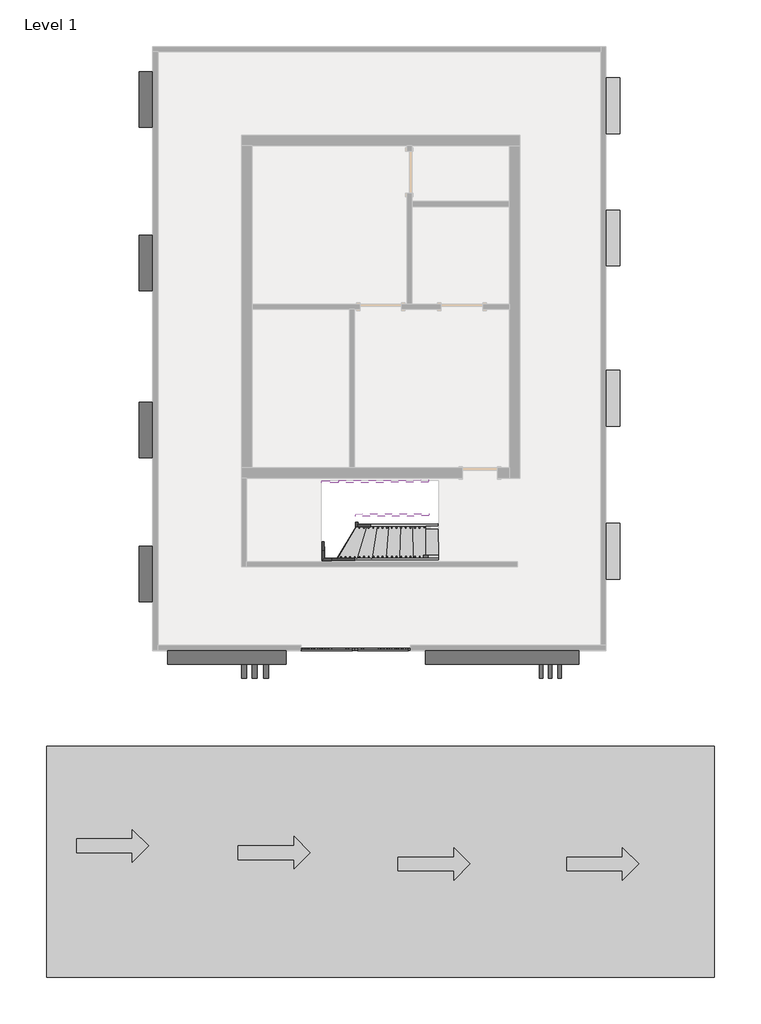
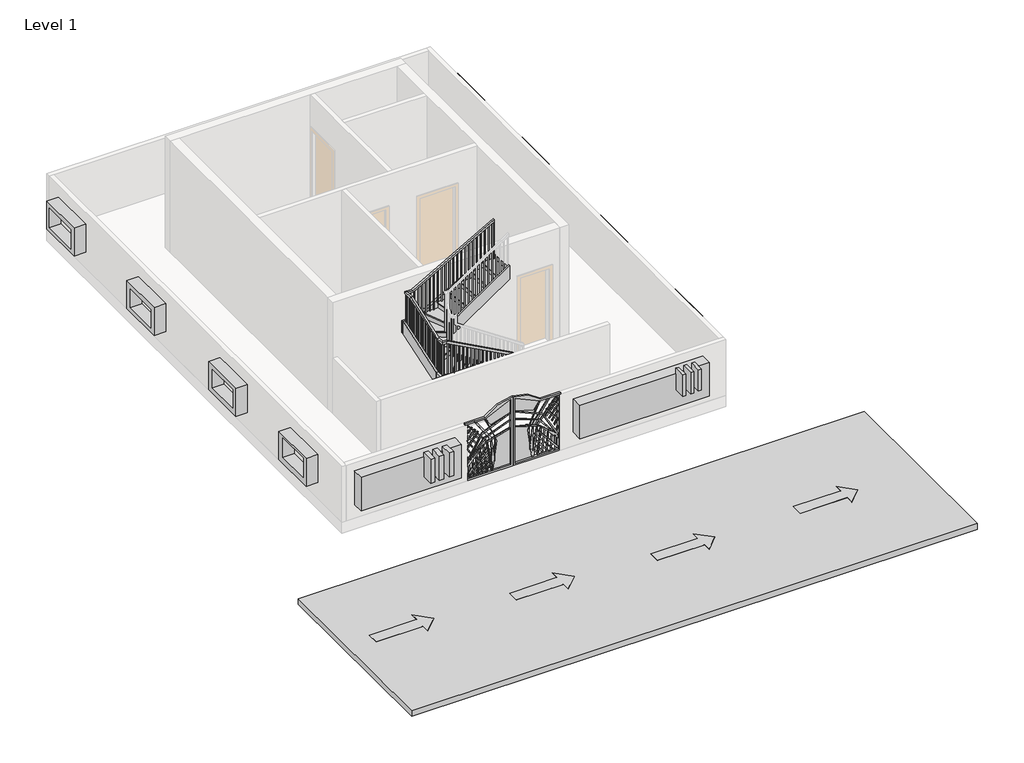
# One storey, part 2 of 2: 9 members, 6 proxies, 4 geographic elements, 1 railing, 1 stair flight.
"""IFC4 building model written with IfcOpenShell, lengths in millimetres."""

from ifc_helpers import new_model, si_unit, frame, origin, place, context, project, spatial, polyline, outline, extrude, faceted_brep, transform, mapped, element, save
from components import generic_models_6bc30956, generic_models_2_generic_models_2_e56ad787, generic_models_3_generic_models_3_7537cf84, generic_models_4_generic_models_4_efd0a726, generic_models_5_generic_models_5_c5eedb73, generic_models_6_generic_models_6_aab6ac76, direction_arrows_straight_direction_arrow_straight_a0d3235c, stair_flight_03031656

model = new_model("IFC4")

# Units and contexts
model_context = context("Model", 3, world=origin())
ifc_project = project(units=[si_unit("LENGTHUNIT", "METRE", prefix="MILLI")], contexts=[model_context])

# Site, building, storey
site = spatial("IfcSite", under=ifc_project)
building = spatial("IfcBuilding", under=site)
storey = spatial("IfcBuildingStorey", under=building, Name="Level 1", Elevation=0.0)

# Proxies
placement = place(None, origin())
generic_models_shape = generic_models_6bc30956(model_context)
element("IfcBuildingElementProxy", 1, Name="Generic Models", at=placement, inside=storey, context=model_context, shape_type="MappedRepresentation", body=[
    mapped(generic_models_shape, transform((-1950.6589614, -6207.4109248, 0.0), x_axis=(1.0, 0.0, 0.0), y_axis=(0.0, 1.0, 0.0), z_axis=(0.0, 0.0, 1.0))),
])
generic_models_2_generic_models_2_shape = generic_models_2_generic_models_2_e56ad787(model_context)
element("IfcBuildingElementProxy", 2, Name="Generic Models 2 : Generic Models 2", ObjectType="Generic Models 2 : Generic Models 2", at=placement, inside=storey, context=model_context, shape_type="MappedRepresentation", body=[
    mapped(generic_models_2_generic_models_2_shape, transform((0.0, 0.0, 0.0), x_axis=(1.0, 0.0, 0.0), y_axis=(0.0, 1.0, 0.0), z_axis=(0.0, 0.0, 1.0))),
])
generic_models_3_generic_models_3_shape = generic_models_3_generic_models_3_7537cf84(model_context)
element("IfcBuildingElementProxy", 3, Name="Generic Models 3 : Generic Models 3", ObjectType="Generic Models 3 : Generic Models 3", at=placement, inside=storey, context=model_context, shape_type="MappedRepresentation", body=[
    mapped(generic_models_3_generic_models_3_shape, transform((0.0, 0.0, 0.0), x_axis=(1.0, 0.0, 0.0), y_axis=(0.0, 1.0, 0.0), z_axis=(0.0, 0.0, 1.0))),
])
generic_models_4_generic_models_4_shape = generic_models_4_generic_models_4_efd0a726(model_context)
element("IfcBuildingElementProxy", 4, Name="Generic Models 4 : Generic Models 4", ObjectType="Generic Models 4 : Generic Models 4", at=placement, inside=storey, context=model_context, shape_type="MappedRepresentation", body=[
    mapped(generic_models_4_generic_models_4_shape, transform((0.0, 0.0, 0.0), x_axis=(1.0, 0.0, 0.0), y_axis=(0.0, 1.0, 0.0), z_axis=(0.0, 0.0, 1.0))),
])
generic_models_5_generic_models_5_shape = generic_models_5_generic_models_5_c5eedb73(model_context)
element("IfcBuildingElementProxy", 5, Name="Generic Models 5 : Generic Models 5", ObjectType="Generic Models 5 : Generic Models 5", at=placement, inside=storey, context=model_context, shape_type="MappedRepresentation", body=[
    mapped(generic_models_5_generic_models_5_shape, transform((0.0, 0.0, 0.0), x_axis=(1.0, 0.0, 0.0), y_axis=(0.0, 1.0, 0.0), z_axis=(0.0, 0.0, 1.0))),
])
generic_models_6_generic_models_6_shape = generic_models_6_generic_models_6_aab6ac76(model_context)
element("IfcBuildingElementProxy", 6, Name="Generic Models 6 : Generic Models 6", ObjectType="Generic Models 6 : Generic Models 6", at=placement, inside=storey, context=model_context, shape_type="MappedRepresentation", body=[
    mapped(generic_models_6_generic_models_6_shape, transform((0.0, 0.0, 0.0), x_axis=(1.0, 0.0, 0.0), y_axis=(0.0, 1.0, 0.0), z_axis=(0.0, 0.0, 1.0))),
])

# Geographic elements
direction_arrows_straight_direction_arrow_straight_shape = direction_arrows_straight_direction_arrow_straight_a0d3235c(model_context)
element("IfcGeographicElement", 7, ObjectType="Direction Arrows - Straight : Direction Arrow - Straight", at=placement, inside=storey, context=model_context, shape_type="MappedRepresentation", body=[
    mapped(direction_arrows_straight_direction_arrow_straight_shape, transform((-8039.1676831, -10535.5511951, 0.0), x_axis=(0.0, -1.0, 0.0), y_axis=(1.0, 0.0, 0.0), z_axis=(0.0, 0.0, 1.0))),
])
element("IfcGeographicElement", 8, ObjectType="Direction Arrows - Straight : Direction Arrow - Straight", at=placement, inside=storey, context=model_context, shape_type="MappedRepresentation", body=[
    mapped(direction_arrows_straight_direction_arrow_straight_shape, transform((-4497.0089614, -10684.1272926, 0.0), x_axis=(0.0, -1.0, 0.0), y_axis=(1.0, 0.0, 0.0), z_axis=(0.0, 0.0, 1.0))),
])
element("IfcGeographicElement", 9, ObjectType="Direction Arrows - Straight : Direction Arrow - Straight", at=placement, inside=storey, context=model_context, shape_type="MappedRepresentation", body=[
    mapped(direction_arrows_straight_direction_arrow_straight_shape, transform((-998.1589614, -10931.1699092, 0.0), x_axis=(0.0, -1.0, 0.0), y_axis=(1.0, 0.0, 0.0), z_axis=(0.0, 0.0, 1.0))),
])
element("IfcGeographicElement", 10, ObjectType="Direction Arrows - Straight : Direction Arrow - Straight", at=placement, inside=storey, context=model_context, shape_type="MappedRepresentation", body=[
    mapped(direction_arrows_straight_direction_arrow_straight_shape, transform((2697.5410386, -10931.1699092, 0.0), x_axis=(0.0, -1.0, 0.0), y_axis=(1.0, 0.0, 0.0), z_axis=(0.0, 0.0, 1.0))),
])

# Members
element("IfcMember", 11, ObjectType="Stringer - 2\" Width", at=placement, inside=storey, context=model_context, shape_type="SweptSolid", body=[
    extrude(outline(polyline([(-106.4787477, -199.0602913), (0.0, 0.0), (2650.4216713, 0.0), (2487.3820108, -304.8), (91.199922, -304.8), (-106.4787477, -199.0602913)])), frame((-116.1777511, -4276.2080688, 225.7492487), z_axis=(-0.006129891180436159, 0.9999812120405644, 0.0), x_axis=(-0.8817595296628619, -0.005405191516664872, 0.4716682263555571)), (0.0, 0.0, 1.0), 50.8),
])
element("IfcMember", 12, ObjectType="Stringer - 2\" Width", at=placement, inside=storey, context=model_context, shape_type="SweptSolid", body=[
    extrude(outline(polyline([(-2453.5237158, -4239.7350599), (-2453.2123174, -4290.5341055), (-2663.1420684, -4291.8209762), (-2612.6544213, -4240.7105322), (-2453.5237158, -4239.7350599)])), frame((0.0, 0.0, 1130.2029558), z_axis=(0.0, 0.0, 1.0), x_axis=(1.0, 0.0, 0.0)), (0.0, 0.0, 1.0), 345.6659817),
])
element("IfcMember", 13, ObjectType="Stringer - 2\" Width", at=placement, inside=storey, context=model_context, shape_type="SweptSolid", body=[
    extrude(outline(polyline([(-2612.6544213, -4240.7105322), (-2663.1420684, -4291.8209762), (-2664.4731567, -4074.6779247), (-2613.6741111, -4074.3665263), (-2612.6544213, -4240.7105322)])), frame((0.0, 0.0, 1130.2029558), z_axis=(0.0, 0.0, 1.0), x_axis=(1.0, 0.0, 0.0)), (0.0, 0.0, 1.0), 345.6659817),
])
element("IfcMember", 14, ObjectType="Stringer - 2\" Width", at=placement, inside=storey, context=model_context, shape_type="SweptSolid", body=[
    extrude(outline(polyline([(-112.9595567, -326.688092), (0.0, 0.0), (1516.7940002, 1e-07), (1565.1210838, -16.7101466), (1457.9394259, -326.6880919), (-112.9595567, -326.688092)])), frame((-2664.4731567, -4074.6779247, 1475.8689375), z_axis=(0.9999812120405643, 0.006129891180436426, 0.0), x_axis=(-0.00579334548330155, 0.945079850136778, 0.32678817912151675)), (0.0, 0.0, 1.0), 50.8),
])
element("IfcMember", 15, ObjectType="Stringer - 2\" Width", at=placement, inside=storey, context=model_context, shape_type="SweptSolid", body=[
    extrude(outline(polyline([(-111.800968, -163.7049666), (0.0, 0.0), (2130.8093531, 0.0), (1922.648686, -304.8000001), (94.7979387, -304.8000001), (-111.800968, -163.7049666)])), frame((-120.6930289, -3539.621908, 198.2391801), z_axis=(-0.006129891180436335, 0.9999812120405644, 0.0), x_axis=(-0.8257797012408892, -0.005062034812924604, 0.5639700885880922)), (0.0, 0.0, 1.0), 50.8),
])
element("IfcMember", 16, ObjectType="Stringer - 2\" Width", at=placement, inside=storey, context=model_context, shape_type="SweptSolid", body=[
    extrude(outline(polyline([(-476.3090819, -288.3824073), (0.0, 0.0), (441.380003, 0.0), (-62.0453256, -304.8), (-466.3690133, -304.8), (-476.3090819, -288.3824073)])), frame((-1931.0711854, -3550.7195376, 1622.3542381), z_axis=(0.9999812120405644, 0.006129891180436036, 0.0), x_axis=(-0.003174799751355551, 0.5179113315223288, 0.8554284150806)), (0.0, 0.0, 1.0), 50.8),
])
element("IfcMember", 17, ObjectType="Stringer - 2\" Width", at=placement, inside=storey, context=model_context, shape_type="SweptSolid", body=[
    extrude(outline(polyline([(205.0123517, -304.8), (0.0, 0.0), (1938.1040339, 0.0), (2143.1163855, -304.8), (205.0123517, -304.8)])), frame((-1932.4724786, -3322.1238325, 1666.9006308), z_axis=(-0.006129891180436482, 0.9999812120405644, 0.0), x_axis=(0.8297505463599373, 0.005086376118722325, 0.5581112430271984)), (0.0, 0.0, 1.0), 50.8),
])
element("IfcMember", 18, ObjectType="Stringer - 2\" Width", at=placement, inside=storey, context=model_context, shape_type="SweptSolid", body=[
    extrude(outline(polyline([(-2673.5739172, -2590.0529496), (-2673.8853157, -2539.253904), (-2303.2697085, -2536.982028), (-2302.9583101, -2587.7810735), (-2673.5739172, -2590.0529496)])), frame((0.0, 0.0, 1649.0329153), z_axis=(0.0, 0.0, 1.0), x_axis=(1.0, 0.0, 0.0)), (0.0, 0.0, 1.0), 322.5063717),
])
element("IfcMember", 19, ObjectType="Stringer - 2\" Width", at=placement, inside=storey, context=model_context, shape_type="SweptSolid", body=[
    extrude(outline(polyline([(155.3220552, -282.6400873), (0.0, 0.0), (2252.6037587, 1e-07), (2407.9258139, -282.6400872), (155.3220552, -282.6400873)])), frame((-2302.9583101, -2587.7810735, 1649.0329153), z_axis=(-0.006129891180436271, 0.9999812120405643, 0.0), x_axis=(0.8763695910030258, 0.005372151158450038, 0.48160926066378773)), (0.0, 0.0, 1.0), 50.8),
])

# Railing
element("IfcRailing", 20, ObjectType="Handrail - Rectangular", at=placement, inside=storey, context=model_context, shape_type="SolidModel", body=[
    faceted_brep([(-116.4891496, -4225.4090232, 1083.7333333), (-116.4891496, -4225.4090232, 1025.9022634), (-116.800548, -4174.6099776, 1025.9022634), (-116.800548, -4174.6099776, 1083.7333333), (-2474.2717021, -4239.8622452, 2366.4653479), (-2487.1954725, -4239.941468, 2315.6653479), (-2487.506871, -4189.1424224, 2315.6653479), (-2474.5831006, -4189.0631997, 2366.4653479), (-2612.6544213, -4240.7105322, 2366.4653479), (-2612.6544213, -4240.7105322, 2315.6653479), (-2562.1667742, -4189.6000881, 2315.6653479), (-2562.1667742, -4189.6000881, 2366.4653479), (-2613.899826, -4037.5452114, 2366.4653479), (-2613.9521428, -4029.010664, 2315.6653479), (-2563.1530973, -4028.6992655, 2315.6653479), (-2563.1007804, -4037.2338129, 2366.4653479), (-2621.180916, -2849.7666717, 2777.1734867), (-2621.2332328, -2841.2321243, 2726.3734867), (-2570.4341872, -2840.9207258, 2726.3734867), (-2570.3818704, -2849.4552732, 2777.1734867), (-2622.7748716, -2589.7415511, 2777.1734867), (-2622.7748716, -2589.7415511, 2726.3734867), (-2571.6644276, -2640.2291982, 2726.3734867), (-2571.6644276, -2640.2291982, 2777.1734867), (-2452.0429693, -2588.6949634, 2777.1734867), (-2438.8245474, -2588.6139344, 2726.3734867), (-2438.513149, -2639.41298, 2726.3734867), (-2451.7315708, -2639.494009, 2777.1734867), (-328.8448754, -2575.6797456, 3962.4), (-328.533477, -2626.4787912, 3962.4), (-328.533477, -2626.4787912, 3904.22112), (-328.8448754, -2575.6797456, 3904.22112)], [[[0, 1, 2, 3]], [[1, 0, 4, 5]], [[2, 1, 5, 6]], [[3, 2, 6, 7]], [[0, 3, 7, 4]], [[5, 4, 8, 9]], [[6, 5, 9, 10]], [[7, 6, 10, 11]], [[4, 7, 11, 8]], [[9, 8, 12, 13]], [[10, 9, 13, 14]], [[11, 10, 14, 15]], [[8, 11, 15, 12]], [[13, 12, 16, 17]], [[14, 13, 17, 18]], [[15, 14, 18, 19]], [[12, 15, 19, 16]], [[17, 16, 20, 21]], [[18, 17, 21, 22]], [[19, 18, 22, 23]], [[16, 19, 23, 20]], [[21, 20, 24, 25]], [[22, 21, 25, 26]], [[23, 22, 26, 27]], [[20, 23, 27, 24]], [[28, 29, 30, 31]], [[25, 24, 28, 31]], [[26, 25, 31, 30]], [[27, 26, 30, 29]], [[24, 27, 29, 28]]]),
    extrude(outline(polyline([(233.9170124, 19.05), (1235.5250403, 19.05), (1235.5250403, 0.0), (223.2829877, 0.0), (233.9170124, 19.05)])), frame((-352.4784362, -2610.7502757, 4114.191707), z_axis=(-0.0061298911804362555, 0.9999812120405644, 0.0), x_axis=(0.0, 0.0, -1.0)), (0.0, 0.0, 1.0), 19.05),
    extrude(outline(polyline([(233.9170123, 19.05), (1178.8102421, 19.05), (1178.8102421, 0.0), (223.2829877, 0.0), (233.9170123, 19.05)])), frame((-454.0765273, -2611.3730726, 4057.4769088), z_axis=(-0.0061298911804362555, 0.9999812120405644, 0.0), x_axis=(0.0, 0.0, -1.0)), (0.0, 0.0, 1.0), 19.05),
    extrude(outline(polyline([(233.9170124, 19.05), (1122.095444, 19.05), (1122.095444, 0.0), (223.2829877, 0.0), (233.9170124, 19.05)])), frame((-555.6746185, -2611.9958696, 4000.7621107), z_axis=(-0.0061298911804362555, 0.9999812120405644, 0.0), x_axis=(0.0, 0.0, -1.0)), (0.0, 0.0, 1.0), 19.05),
    extrude(outline(polyline([(233.9170123, 19.05), (1234.7139792, 19.05), (1234.7139792, 0.0), (223.2829877, 0.0), (233.9170123, 19.05)])), frame((-657.2727096, -2612.6186665, 3944.0473125), z_axis=(-0.0061298911804362555, 0.9999812120405644, 0.0), x_axis=(0.0, 0.0, -1.0)), (0.0, 0.0, 1.0), 19.05),
    extrude(outline(polyline([(233.9170123, 19.05), (1177.999181, 19.05), (1177.999181, 0.0), (223.2829876, 0.0), (233.9170123, 19.05)])), frame((-758.8708008, -2613.2414635, 3887.3325143), z_axis=(-0.0061298911804362555, 0.9999812120405644, 0.0), x_axis=(0.0, 0.0, -1.0)), (0.0, 0.0, 1.0), 19.05),
    extrude(outline(polyline([(233.9170123, 19.05), (1121.2843829, 19.05), (1121.2843829, 0.0), (223.2829877, 0.0), (233.9170123, 19.05)])), frame((-860.4688919, -2613.8642604, 3830.6177162), z_axis=(-0.0061298911804362555, 0.9999812120405644, 0.0), x_axis=(0.0, 0.0, -1.0)), (0.0, 0.0, 1.0), 19.05),
    extrude(outline(polyline([(233.9170123, 19.0499999), (1233.902918, 19.0499999), (1233.902918, 0.0), (223.2829876, 0.0), (233.9170123, 19.0499999)])), frame((-962.0669831, -2614.4870574, 3773.902918), z_axis=(-0.0061298911804362555, 0.9999812120405644, 0.0), x_axis=(0.0, 0.0, -1.0)), (0.0, 0.0, 1.0), 19.05),
    extrude(outline(polyline([(233.9170123, 19.05), (1177.1881199, 19.05), (1177.1881199, 0.0), (223.2829877, 0.0), (233.9170123, 19.05)])), frame((-1063.6650742, -2615.1098543, 3717.1881199), z_axis=(-0.0061298911804362555, 0.9999812120405644, 0.0), x_axis=(0.0, 0.0, -1.0)), (0.0, 0.0, 1.0), 19.05),
    extrude(outline(polyline([(233.9170123, 19.05), (1120.4733217, 19.05), (1120.4733217, 0.0), (223.2829876, 0.0), (233.9170123, 19.05)])), frame((-1165.2631653, -2615.7326513, 3660.4733217), z_axis=(-0.0061298911804362555, 0.9999812120405644, 0.0), x_axis=(0.0, 0.0, -1.0)), (0.0, 0.0, 1.0), 19.05),
    extrude(outline(polyline([(233.9170123, 19.05), (1233.0918569, 19.05), (1233.0918569, 0.0), (223.2829877, 0.0), (233.9170123, 19.05)])), frame((-1266.8612565, -2616.3554482, 3603.7585236), z_axis=(-0.0061298911804362555, 0.9999812120405644, 0.0), x_axis=(0.0, 0.0, -1.0)), (0.0, 0.0, 1.0), 19.05),
    extrude(outline(polyline([(233.9170123, 19.05), (1176.3770587, 19.05), (1176.3770587, 0.0), (223.2829876, 0.0), (233.9170123, 19.05)])), frame((-1368.4593476, -2616.9782451, 3547.0437254), z_axis=(-0.0061298911804362555, 0.9999812120405644, 0.0), x_axis=(0.0, 0.0, -1.0)), (0.0, 0.0, 1.0), 19.05),
    extrude(outline(polyline([(233.9170123, 19.05), (1288.995594, 19.05), (1288.995594, 0.0), (223.2829877, 0.0), (233.9170123, 19.05)])), frame((-1470.0574388, -2617.6010421, 3490.3289273), z_axis=(-0.0061298911804362555, 0.9999812120405644, 0.0), x_axis=(0.0, 0.0, -1.0)), (0.0, 0.0, 1.0), 19.05),
    extrude(outline(polyline([(233.9170123, 19.05), (1232.2807958, 19.05), (1232.2807958, 0.0), (223.2829876, 0.0), (233.9170123, 19.05)])), frame((-1571.6555299, -2618.223839, 3433.6141291), z_axis=(-0.0061298911804362555, 0.9999812120405644, 0.0), x_axis=(0.0, 0.0, -1.0)), (0.0, 0.0, 1.0), 19.05),
    extrude(outline(polyline([(233.9170123, 19.05), (1175.5659977, 19.05), (1175.5659977, 0.0), (223.2829877, 0.0), (233.9170123, 19.05)])), frame((-1673.2536211, -2618.846636, 3376.899331), z_axis=(-0.0061298911804362555, 0.9999812120405644, 0.0), x_axis=(0.0, 0.0, -1.0)), (0.0, 0.0, 1.0), 19.05),
    extrude(outline(polyline([(233.9170123, 19.05), (1118.8511995, 19.05), (1118.8511995, 0.0), (223.2829876, 0.0), (233.9170123, 19.05)])), frame((-1774.8517122, -2619.4694329, 3320.1845328), z_axis=(-0.0061298911804362555, 0.9999812120405644, 0.0), x_axis=(0.0, 0.0, -1.0)), (0.0, 0.0, 1.0), 19.05),
    extrude(outline(polyline([(233.9170123, 19.05), (1231.4697347, 19.05), (1231.4697347, 0.0), (223.2829877, 0.0), (233.9170123, 19.05)])), frame((-1876.4498033, -2620.0922299, 3263.4697347), z_axis=(-0.0061298911804362555, 0.9999812120405644, 0.0), x_axis=(0.0, 0.0, -1.0)), (0.0, 0.0, 1.0), 19.05),
    extrude(outline(polyline([(233.9170123, 19.05), (1174.7549365, 19.05), (1174.7549365, 0.0), (223.2829876, 0.0), (233.9170123, 19.05)])), frame((-1978.0478945, -2620.7150268, 3206.7549365), z_axis=(-0.0061298911804362555, 0.9999812120405644, 0.0), x_axis=(0.0, 0.0, -1.0)), (0.0, 0.0, 1.0), 19.05),
    extrude(outline(polyline([(233.9170124, 19.05), (1118.0401384, 19.05), (1118.0401384, 0.0), (223.2829877, 0.0), (233.9170124, 19.05)])), frame((-2079.6459856, -2621.3378238, 3150.0401384), z_axis=(-0.0061298911804362555, 0.9999812120405644, 0.0), x_axis=(0.0, 0.0, -1.0)), (0.0, 0.0, 1.0), 19.05),
    extrude(outline(polyline([(233.9170123, 19.05), (1230.6586735, 19.05), (1230.6586735, 0.0), (223.2829876, 0.0), (233.9170123, 19.05)])), frame((-2181.2440768, -2621.9606207, 3093.3253402), z_axis=(-0.0061298911804362555, 0.9999812120405644, 0.0), x_axis=(0.0, 0.0, -1.0)), (0.0, 0.0, 1.0), 19.05),
    extrude(outline(polyline([(233.9170124, 19.05), (1173.9438754, 19.05), (1173.9438754, 0.0), (223.2829877, 0.0), (233.9170124, 19.05)])), frame((-2282.8421679, -2622.5834176, 3036.6105421), z_axis=(-0.0061298911804362555, 0.9999812120405644, 0.0), x_axis=(0.0, 0.0, -1.0)), (0.0, 0.0, 1.0), 19.05),
    extrude(outline(polyline([(233.9170123, 19.05), (1117.2290772, 19.05), (1117.2290772, 0.0), (223.2829877, 0.0), (233.9170123, 19.05)])), frame((-2384.4402591, -2623.2062146, 2979.8957439), z_axis=(-0.0061298911804362555, 0.9999812120405644, 0.0), x_axis=(0.0, 0.0, -1.0)), (0.0, 0.0, 1.0), 19.05),
    extrude(outline(polyline([(-2505.2047667, -2604.8961439), (-2486.1551246, -2604.7793694), (-2486.0383502, -2623.8290115), (-2505.0879923, -2623.945786), (-2505.2047667, -2604.8961439)])), frame((0.0, 0.0, 1862.6666667), z_axis=(0.0, 0.0, 1.0), x_axis=(1.0, 0.0, 0.0)), (0.0, 0.0, 1.0), 863.70682),
    extrude(outline(polyline([(-2606.2189857, -2700.7671513), (-2606.3357602, -2681.7175092), (-2587.2861181, -2681.6007347), (-2587.1693436, -2700.6503768), (-2606.2189857, -2700.7671513)])), frame((0.0, 0.0, 1862.6666667), z_axis=(0.0, 0.0, 1.0), x_axis=(1.0, 0.0, 0.0)), (0.0, 0.0, 1.0), 863.70682),
    extrude(outline(polyline([(-2605.5961888, -2802.3652424), (-2605.7129632, -2783.3156003), (-2586.6633211, -2783.1988259), (-2586.5465467, -2802.248468), (-2605.5961888, -2802.3652424)])), frame((0.0, 0.0, 1862.6666667), z_axis=(0.0, 0.0, 1.0), x_axis=(1.0, 0.0, 0.0)), (0.0, 0.0, 1.0), 863.70682),
    extrude(outline(polyline([(225.3065228, 19.0499999), (1243.2088863, 19.0499999), (1243.2088863, 0.0), (231.8934772, 0.0), (225.3065228, 19.0499999)])), frame((-2604.9733918, -2903.9633335, 2936.5422196), z_axis=(0.9999812120405643, 0.0061298911804362685, 0.0), x_axis=(0.0, 0.0, -1.0)), (0.0, 0.0, 1.0), 19.05),
    extrude(outline(polyline([(225.3065229, 19.05), (1208.078463, 19.05), (1208.078463, 0.0), (231.8934772, 0.0), (225.3065229, 19.05)])), frame((-2604.3505949, -3005.5614247, 2901.4117963), z_axis=(0.9999812120405643, 0.0061298911804362685, 0.0), x_axis=(0.0, 0.0, -1.0)), (0.0, 0.0, 1.0), 19.05),
    extrude(outline(polyline([(225.3065228, 19.05), (1172.9480396, 19.05), (1172.9480396, 0.0), (231.8934772, 0.0), (225.3065228, 19.05)])), frame((-2603.727798, -3107.1595158, 2866.2813729), z_axis=(0.9999812120405643, 0.0061298911804362685, 0.0), x_axis=(0.0, 0.0, -1.0)), (0.0, 0.0, 1.0), 19.05),
    extrude(outline(polyline([(225.3065228, 19.05), (1137.8176163, 19.05), (1137.8176163, 0.0), (231.8934772, 0.0), (225.3065228, 19.05)])), frame((-2603.105001, -3208.757607, 2831.1509496), z_axis=(0.9999812120405643, 0.0061298911804362685, 0.0), x_axis=(0.0, 0.0, -1.0)), (0.0, 0.0, 1.0), 19.05),
    extrude(outline(polyline([(225.3065228, 19.05), (1102.687193, 19.05), (1102.687193, 0.0), (231.8934772, 0.0), (225.3065228, 19.05)])), frame((-2602.4822041, -3310.3556981, 2796.0205263), z_axis=(0.9999812120405643, 0.0061298911804362685, 0.0), x_axis=(0.0, 0.0, -1.0)), (0.0, 0.0, 1.0), 19.05),
    extrude(outline(polyline([(225.3065228, 19.05), (1236.890103, 19.05), (1236.890103, 0.0), (231.8934772, 0.0), (225.3065228, 19.05)])), frame((-2601.8594071, -3411.9537893, 2760.890103), z_axis=(0.9999812120405643, 0.0061298911804362685, 0.0), x_axis=(0.0, 0.0, -1.0)), (0.0, 0.0, 1.0), 19.05),
    extrude(outline(polyline([(225.3065229, 19.05), (1201.7596797, 19.05), (1201.7596797, 0.0), (231.8934772, 0.0), (225.3065229, 19.05)])), frame((-2601.2366102, -3513.5518804, 2725.7596797), z_axis=(0.9999812120405643, 0.0061298911804362685, 0.0), x_axis=(0.0, 0.0, -1.0)), (0.0, 0.0, 1.0), 19.05),
    extrude(outline(polyline([(225.3065228, 19.0499999), (1166.6292563, 19.0499999), (1166.6292563, 0.0), (231.8934772, 0.0), (225.3065228, 19.0499999)])), frame((-2600.6138132, -3615.1499715, 2690.6292563), z_axis=(0.9999812120405643, 0.0061298911804362685, 0.0), x_axis=(0.0, 0.0, -1.0)), (0.0, 0.0, 1.0), 19.05),
    extrude(outline(polyline([(225.3065228, 19.05), (1131.498833, 19.05), (1131.498833, 0.0), (231.8934772, 0.0), (225.3065228, 19.05)])), frame((-2599.9910163, -3716.7480627, 2655.498833), z_axis=(0.9999812120405643, 0.0061298911804362685, 0.0), x_axis=(0.0, 0.0, -1.0)), (0.0, 0.0, 1.0), 19.05),
    extrude(outline(polyline([(225.3065228, 19.05), (1096.3684097, 19.05), (1096.3684097, 0.0), (231.8934772, 0.0), (225.3065228, 19.05)])), frame((-2599.3682194, -3818.3461538, 2620.3684097), z_axis=(0.9999812120405643, 0.0061298911804362685, 0.0), x_axis=(0.0, 0.0, -1.0)), (0.0, 0.0, 1.0), 19.05),
    extrude(outline(polyline([(225.3065228, 19.05), (1230.5713197, 19.05), (1230.5713197, 0.0), (231.8934772, 0.0), (225.3065228, 19.05)])), frame((-2598.7454224, -3919.944245, 2585.2379864), z_axis=(0.9999812120405643, 0.0061298911804362685, 0.0), x_axis=(0.0, 0.0, -1.0)), (0.0, 0.0, 1.0), 19.05),
    extrude(outline(polyline([(225.3065228, 19.05), (1195.4408963, 19.05), (1195.4408963, 0.0), (231.8934771, 0.0), (225.3065228, 19.05)])), frame((-2598.1226255, -4021.5423361, 2550.107563), z_axis=(0.9999812120405643, 0.0061298911804362685, 0.0), x_axis=(0.0, 0.0, -1.0)), (0.0, 0.0, 1.0), 19.05),
    extrude(outline(polyline([(-2597.4998285, -4123.1404273), (-2597.6166029, -4104.0907852), (-2578.5669609, -4103.9740107), (-2578.4501864, -4123.0236528), (-2597.4998285, -4123.1404273)])), frame((0.0, 0.0, 1354.6666667), z_axis=(0.0, 0.0, 1.0), x_axis=(1.0, 0.0, 0.0)), (0.0, 0.0, 1.0), 960.9986813),
    extrude(outline(polyline([(-2545.415828, -4224.4230609), (-2564.4654701, -4224.5398353), (-2564.5822445, -4205.4901932), (-2545.5326024, -4205.3734188), (-2545.415828, -4224.4230609)])), frame((0.0, 0.0, 1354.6666667), z_axis=(0.0, 0.0, 1.0), x_axis=(1.0, 0.0, 0.0)), (0.0, 0.0, 1.0), 960.9986813),
    extrude(outline(polyline([(223.4181002, 19.05), (1171.1283424, 19.05), (1171.1283424, 0.0), (233.7818998, 0.0), (223.4181002, 19.05)])), frame((-2443.8177368, -4223.800264, 2525.7950091), z_axis=(-0.006129891180436165, 0.9999812120405643, 0.0), x_axis=(0.0, 0.0, -1.0)), (0.0, 0.0, 1.0), 19.05),
    extrude(outline(polyline([(223.4181002, 19.05), (1115.8547448, 19.05), (1115.8547448, 0.0), (233.7818998, 0.0), (223.4181002, 19.05)])), frame((-2342.2196457, -4223.177467, 2470.5214115), z_axis=(-0.006129891180436165, 0.9999812120405643, 0.0), x_axis=(0.0, 0.0, -1.0)), (0.0, 0.0, 1.0), 19.05),
    extrude(outline(polyline([(223.4181002, 19.05), (1229.9144805, 19.05), (1229.9144805, 0.0), (233.7818997, 0.0), (223.4181002, 19.05)])), frame((-2240.6215545, -4222.5546701, 2415.2478138), z_axis=(-0.006129891180436165, 0.9999812120405643, 0.0), x_axis=(0.0, 0.0, -1.0)), (0.0, 0.0, 1.0), 19.05),
    extrude(outline(polyline([(223.4181002, 19.05), (1174.6408829, 19.05), (1174.6408829, 0.0), (233.7818998, 0.0), (223.4181002, 19.05)])), frame((-2139.0234634, -4221.9318731, 2359.9742162), z_axis=(-0.006129891180436165, 0.9999812120405643, 0.0), x_axis=(0.0, 0.0, -1.0)), (0.0, 0.0, 1.0), 19.05),
    extrude(outline(polyline([(223.4181003, 19.0499999), (1119.3672853, 19.0499999), (1119.3672853, 0.0), (233.7818998, 0.0), (223.4181003, 19.0499999)])), frame((-2037.4253723, -4221.3090762, 2304.7006186), z_axis=(-0.006129891180436165, 0.9999812120405643, 0.0), x_axis=(0.0, 0.0, -1.0)), (0.0, 0.0, 1.0), 19.05),
    extrude(outline(polyline([(223.4181002, 19.05), (1064.0936876, 19.05), (1064.0936876, 0.0), (233.7818998, 0.0), (223.4181002, 19.05)])), frame((-1935.8272811, -4220.6862792, 2249.4270209), z_axis=(-0.006129891180436165, 0.9999812120405643, 0.0), x_axis=(0.0, 0.0, -1.0)), (0.0, 0.0, 1.0), 19.05),
    extrude(outline(polyline([(223.4181002, 19.05), (1178.1534233, 19.05), (1178.1534233, 0.0), (233.7818998, 0.0), (223.4181002, 19.05)])), frame((-1834.22919, -4220.0634823, 2194.1534233), z_axis=(-0.006129891180436165, 0.9999812120405643, 0.0), x_axis=(0.0, 0.0, -1.0)), (0.0, 0.0, 1.0), 19.05),
    extrude(outline(polyline([(223.4181002, 19.05), (1122.8798256, 19.05), (1122.8798256, 0.0), (233.7818997, 0.0), (223.4181002, 19.05)])), frame((-1732.6310988, -4219.4406854, 2138.8798256), z_axis=(-0.006129891180436165, 0.9999812120405643, 0.0), x_axis=(0.0, 0.0, -1.0)), (0.0, 0.0, 1.0), 19.05),
    extrude(outline(polyline([(223.4181002, 19.05), (1067.606228, 19.05), (1067.606228, 0.0), (233.7818998, 0.0), (223.4181002, 19.05)])), frame((-1631.0330077, -4218.8178884, 2083.606228), z_axis=(-0.006129891180436165, 0.9999812120405643, 0.0), x_axis=(0.0, 0.0, -1.0)), (0.0, 0.0, 1.0), 19.05),
    extrude(outline(polyline([(223.4181003, 19.05), (1181.6659637, 19.05), (1181.6659637, 0.0), (233.7818998, 0.0), (223.4181003, 19.05)])), frame((-1529.4349165, -4218.1950915, 2028.3326304), z_axis=(-0.006129891180436165, 0.9999812120405643, 0.0), x_axis=(0.0, 0.0, -1.0)), (0.0, 0.0, 1.0), 19.05),
    extrude(outline(polyline([(223.4181002, 19.05), (1126.392366, 19.05), (1126.392366, 0.0), (233.7818998, 0.0), (223.4181002, 19.05)])), frame((-1427.8368254, -4217.5722945, 1973.0590327), z_axis=(-0.006129891180436165, 0.9999812120405643, 0.0), x_axis=(0.0, 0.0, -1.0)), (0.0, 0.0, 1.0), 19.05),
    extrude(outline(polyline([(223.4181002, 19.0499999), (1071.1187684, 19.0499999), (1071.1187684, 0.0), (233.7818998, 0.0), (223.4181002, 19.0499999)])), frame((-1326.2387343, -4216.9494976, 1917.7854351), z_axis=(-0.006129891180436165, 0.9999812120405643, 0.0), x_axis=(0.0, 0.0, -1.0)), (0.0, 0.0, 1.0), 19.05),
    extrude(outline(polyline([(223.4181002, 19.05), (1185.1785041, 19.05), (1185.1785041, 0.0), (233.7818997, 0.0), (223.4181002, 19.05)])), frame((-1224.6406431, -4216.3267006, 1862.5118374), z_axis=(-0.006129891180436165, 0.9999812120405643, 0.0), x_axis=(0.0, 0.0, -1.0)), (0.0, 0.0, 1.0), 19.05),
    extrude(outline(polyline([(223.4181002, 19.05), (1129.9049065, 19.05), (1129.9049065, 0.0), (233.7818998, 0.0), (223.4181002, 19.05)])), frame((-1123.042552, -4215.7039037, 1807.2382398), z_axis=(-0.006129891180436165, 0.9999812120405643, 0.0), x_axis=(0.0, 0.0, -1.0)), (0.0, 0.0, 1.0), 19.05),
    extrude(outline(polyline([(223.4181003, 19.05), (1074.6313089, 19.05), (1074.6313089, 0.0), (233.7818998, 0.0), (223.4181003, 19.05)])), frame((-1021.4444608, -4215.0811067, 1751.9646422), z_axis=(-0.006129891180436165, 0.9999812120405643, 0.0), x_axis=(0.0, 0.0, -1.0)), (0.0, 0.0, 1.0), 19.05),
    extrude(outline(polyline([(223.4181002, 19.05), (1188.6910445, 19.05), (1188.6910445, 0.0), (233.7818998, 0.0), (223.4181002, 19.05)])), frame((-919.8463697, -4214.4583098, 1696.6910445), z_axis=(-0.006129891180436165, 0.9999812120405643, 0.0), x_axis=(0.0, 0.0, -1.0)), (0.0, 0.0, 1.0), 19.05),
    extrude(outline(polyline([(223.4181002, 19.05), (1133.4174469, 19.05), (1133.4174469, 0.0), (233.7818998, 0.0), (223.4181002, 19.05)])), frame((-818.2482785, -4213.8355129, 1641.4174469), z_axis=(-0.006129891180436165, 0.9999812120405643, 0.0), x_axis=(0.0, 0.0, -1.0)), (0.0, 0.0, 1.0), 19.05),
    extrude(outline(polyline([(223.4181002, 19.05), (1078.1438492, 19.05), (1078.1438492, 0.0), (233.7818997, 0.0), (223.4181002, 19.05)])), frame((-716.6501874, -4213.2127159, 1586.1438492), z_axis=(-0.006129891180436165, 0.9999812120405643, 0.0), x_axis=(0.0, 0.0, -1.0)), (0.0, 0.0, 1.0), 19.05),
    extrude(outline(polyline([(223.4181002, 19.0499999), (1192.2035849, 19.0499999), (1192.2035849, 0.0), (233.7818998, 0.0), (223.4181002, 19.0499999)])), frame((-615.0520963, -4212.589919, 1530.8702516), z_axis=(-0.006129891180436165, 0.9999812120405643, 0.0), x_axis=(0.0, 0.0, -1.0)), (0.0, 0.0, 1.0), 19.05),
    extrude(outline(polyline([(223.4181003, 19.05), (1136.9299873, 19.05), (1136.9299873, 0.0), (233.7818998, 0.0), (223.4181003, 19.05)])), frame((-513.4540051, -4211.967122, 1475.596654), z_axis=(-0.006129891180436165, 0.9999812120405643, 0.0), x_axis=(0.0, 0.0, -1.0)), (0.0, 0.0, 1.0), 19.05),
    extrude(outline(polyline([(223.4181002, 19.05), (1081.6563896, 19.05), (1081.6563896, 0.0), (233.7818998, 0.0), (223.4181002, 19.05)])), frame((-411.855914, -4211.3443251, 1420.3230563), z_axis=(-0.006129891180436165, 0.9999812120405643, 0.0), x_axis=(0.0, 0.0, -1.0)), (0.0, 0.0, 1.0), 19.05),
    extrude(outline(polyline([(223.4181002, 19.05), (1195.7161254, 19.05), (1195.7161254, 0.0), (233.7818998, 0.0), (223.4181002, 19.05)])), frame((-310.2578228, -4210.7215281, 1365.0494587), z_axis=(-0.006129891180436165, 0.9999812120405643, 0.0), x_axis=(0.0, 0.0, -1.0)), (0.0, 0.0, 1.0), 19.05),
    extrude(outline(polyline([(223.4181002, 19.05), (1140.4425277, 19.05), (1140.4425277, 0.0), (233.7818997, 0.0), (223.4181002, 19.05)])), frame((-208.6597317, -4210.0987312, 1309.775861), z_axis=(-0.006129891180436165, 0.9999812120405643, 0.0), x_axis=(0.0, 0.0, -1.0)), (0.0, 0.0, 1.0), 19.05),
    extrude(outline(polyline([(-2606.6860834, -2624.5685829), (-2606.8028579, -2605.5189408), (-2587.7532158, -2605.4021664), (-2587.6364414, -2624.4518085), (-2606.6860834, -2624.5685829)])), frame((0.0, 0.0, 1862.6666667), z_axis=(0.0, 0.0, 1.0), x_axis=(1.0, 0.0, 0.0)), (0.0, 0.0, 1.0), 863.70682),
    extrude(outline(polyline([(-2577.8273895, -4224.621744), (-2596.8770316, -4224.7385184), (-2596.993806, -4205.6888763), (-2577.9441639, -4205.5721019), (-2577.8273895, -4224.621744)])), frame((0.0, 0.0, 1354.6666667), z_axis=(0.0, 0.0, 1.0), x_axis=(1.0, 0.0, 0.0)), (0.0, 0.0, 1.0), 960.9986813),
    extrude(outline(polyline([(233.9170123, 19.05), (1248.8374409, 19.05), (1248.8374409, 0.0), (223.2829876, 0.0), (233.9170123, 19.05)])), frame((-328.630789, -2610.6040895, 4127.5041076), z_axis=(-0.0061298911804362555, 0.9999812120405644, 0.0), x_axis=(0.0, 0.0, -1.0)), (0.0, 0.0, 1.0), 19.05),
    extrude(outline(polyline([(223.4181002, 19.05), (1090.3508299, 19.05), (1090.3508299, 0.0), (233.7818998, 0.0), (223.4181002, 19.05)])), frame((-116.5864616, -4209.5343215, 1259.6841632), z_axis=(-0.006129891180436165, 0.9999812120405643, 0.0), x_axis=(0.0, 0.0, -1.0)), (0.0, 0.0, 1.0), 19.05),
])

# Stair flight
stair_flight_shape = stair_flight_03031656(model_context)
element("IfcStairFlight", 21, ObjectType="2\" Tread 1\" Nosing 1/4\" Riser", at=placement, inside=storey, context=model_context, shape_type="MappedRepresentation", body=[
    mapped(stair_flight_shape, transform((0.0, 0.0, 0.0), x_axis=(1.0, 0.0, 0.0), y_axis=(0.0, 1.0, 0.0), z_axis=(0.0, 0.0, 1.0))),
])

save(model, "model.ifc")

# Revit data of these elements
# Type
#   m.s. sheet = none
#   2" x2" pipe = none
#   1"x1"pipe = none
#   Default Elevation = 0
# Type "Handrail - Rectangular"
#   Assembly Code = "C2010400"
#   built-in parameter 1008612 = 0.0416667 (stored number, unit not read)
#   built-in parameter 1008611 = 0.0416667 (stored number, unit not read)
#   built-in parameter 1008609 = 0.333333 (stored number, unit not read)
#   built-in parameter 1008604 = 0.166667 (stored number, unit not read)
#   built-in parameter 1008603 = 0.166667 (stored number, unit not read)
#   Railing Height = 3' - 0"
#   built-in parameter 1008630 = 2
#   built-in parameter 1008610 = 2
#   built-in parameter 1008618 = Baluster - Square : 3/4"
# Element 1 (IfcBuildingElementProxy)
#   Phase Created = New Construction
#   Materials on its faces: "r1"
# Element 2 (IfcBuildingElementProxy, "Generic Models 2 : Generic Models 2")
#   Phase Created = New Construction
#   Materials on its faces: "Laminate, Ivory, Matte"
# Element 3 (IfcBuildingElementProxy, "Generic Models 3 : Generic Models 3")
#   Phase Created = New Construction
# Element 4 (IfcBuildingElementProxy, "Generic Models 4 : Generic Models 4")
#   Phase Created = New Construction
#   Materials on its faces: "Parking Stripe"
# Element 5 (IfcBuildingElementProxy, "Generic Models 5 : Generic Models 5")
#   Phase Created = New Construction
#   Materials on its faces: "Parking Stripe"
# Element 6 (IfcBuildingElementProxy, "Generic Models 6 : Generic Models 6")
#   Phase Created = New Construction
#   Materials on its faces: "Parking Stripe"
# Elements 7, 8, 9, 10 (IfcGeographicElement, "Direction Arrows - Straight : Direction Arrow - Straight")
#   Phase Created = New Construction
#   Materials on its faces: "Paint - White"
# Elements 11, 12, 13, 14, 15, 16, 17, 18, 19 (IfcMember, "Stringer - 2\" Width")
#   Phase Created = New Construction
# Element 20 (IfcRailing, "Handrail - Rectangular")
#   Phase Created = New Construction
# Element 21 (IfcStairFlight, "2\" Tread 1\" Nosing 1/4\" Riser")
#   Phase Created = New Construction
# Materials
#   "r1": class "Generic", colour RGB 120 120 120, transparency 0, Cost = 0
#   "Laminate, Ivory, Matte": class "Plastic", colour RGB 247 247 239, transparency 0, Description = "Plastic Laminate - Ivory, Matte", Cost = 0
#   "Parking Stripe": class "Paint", colour RGB 250 250 91, transparency 0, Cost = 0
#   "Paint - White": class "Paint", colour RGB 249 249 249, transparency 0
